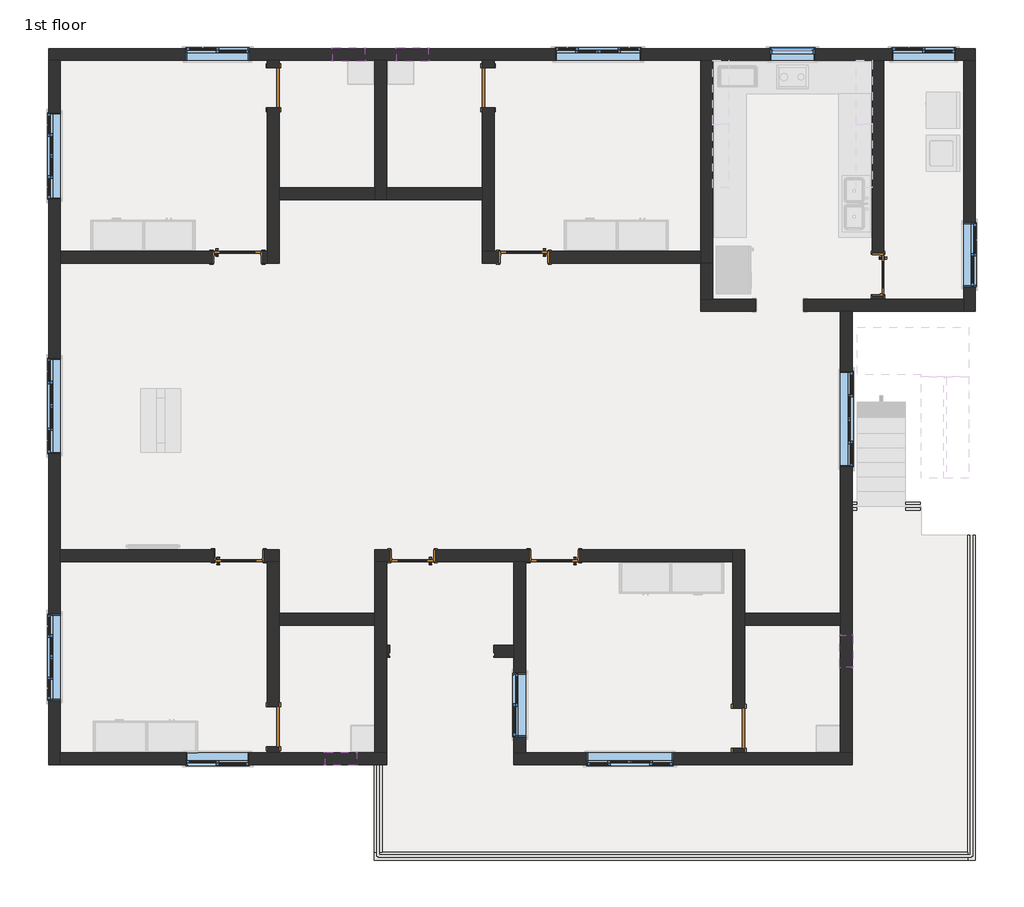
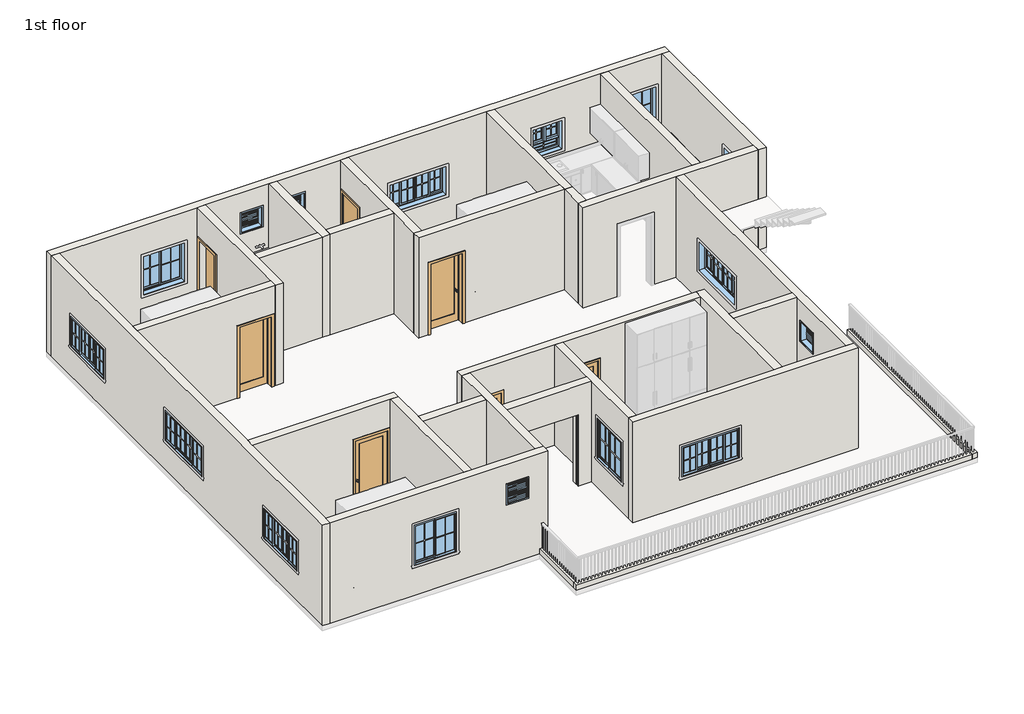
# One storey, part 1 of 4: 31 walls, 16 windows, 10 doors.
"""IFC4 building model written with IfcOpenShell, lengths in millimetres."""

from ifc_helpers import new_model, si_unit, frame, origin, place, context, project, spatial, polyline, outline, extrude, faceted_brep, transform, mapped, element, save
from components import door_ac3c0746, door_868ee8a9, door_3b97b8e7, door_c0815308, door_5e1232af, door_bb98abfd, window_ced37e8f, window_f2d8fef0, window_5af5dca6, window_95c4569f, window_58cce754

model = new_model("IFC4")

# Units and contexts
model_context = context("Model", 3, world=origin())
ifc_project = project(units=[si_unit("LENGTHUNIT", "METRE", prefix="MILLI")], contexts=[model_context])

# Site, building, storey
site = spatial("IfcSite", under=ifc_project)
building = spatial("IfcBuilding", under=site)
storey = spatial("IfcBuildingStorey", under=building, Name="1st floor", Elevation=3810.0)

# Doors
placement = place(None, origin())
door_shape = door_ac3c0746(model_context)
element("IfcDoor", 1, ObjectType="Door-Interior-Single-1_Panel-Wood : 30\" x 84\"", at=placement, inside=storey, context=model_context, shape_type="MappedRepresentation", body=[
    mapped(door_shape, transform((7861.3010838, 2743.2660813, 3810.0), x_axis=(0.0, -1.0, 0.0), y_axis=(1.0, 0.0, 0.0), z_axis=(0.0, 0.0, 1.0))),
])
door_2_shape = door_868ee8a9(model_context)
element("IfcDoor", 2, ObjectType="Door-Interior-Single-1_Panel-Wood : 36\" x 84\"", at=placement, inside=storey, context=model_context, shape_type="MappedRepresentation", body=[
    mapped(door_2_shape, transform((1076.3260838, 3076.6410813, 3810.0), x_axis=(-1.0, 0.0, 0.0), y_axis=(0.0, -1.0, 0.0), z_axis=(0.0, 0.0, 1.0))),
])
element("IfcDoor", 3, ObjectType="Door-Interior-Single-1_Panel-Wood : 36\" x 84\"", at=placement, inside=storey, context=model_context, shape_type="MappedRepresentation", body=[
    mapped(door_2_shape, transform((-4384.6739162, -2644.7089187, 3810.0), x_axis=(1.0, 0.0, 0.0), y_axis=(0.0, 1.0, 0.0), z_axis=(0.0, 0.0, 1.0))),
])
door_3_shape = door_3b97b8e7(model_context)
element("IfcDoor", 4, ObjectType="Door-Interior-Single-1_Panel-Wood : 36\" x 84\"", at=placement, inside=storey, context=model_context, shape_type="MappedRepresentation", body=[
    mapped(door_3_shape, transform((1660.5260838, -2644.7089187, 3810.0), x_axis=(-1.0, 0.0, 0.0), y_axis=(0.0, -1.0, 0.0), z_axis=(0.0, 0.0, 1.0))),
])
element("IfcDoor", 5, ObjectType="Door-Interior-Single-1_Panel-Wood : 36\" x 84\"", at=placement, inside=storey, context=model_context, shape_type="MappedRepresentation", body=[
    mapped(door_3_shape, transform((-4410.0739162, 3076.6410813, 3810.0), x_axis=(1.0, 0.0, 0.0), y_axis=(0.0, 1.0, 0.0), z_axis=(0.0, 0.0, 1.0))),
])
door_4_shape = door_c0815308(model_context)
element("IfcDoor", 6, ObjectType="Door-Interior-Single-Full Glass-Wood : 32\" x 84\"", at=placement, inside=storey, context=model_context, shape_type="MappedRepresentation", body=[
    mapped(door_4_shape, transform((-1057.2739162, -2644.7089187, 3810.0), x_axis=(-1.0, 0.0, 0.0), y_axis=(0.0, -1.0, 0.0), z_axis=(0.0, 0.0, 1.0))),
])
door_5_shape = door_5e1232af(model_context)
element("IfcDoor", 7, ObjectType="Single-Flush : 30\" x 84\"", at=placement, inside=storey, context=model_context, shape_type="MappedRepresentation", body=[
    mapped(door_5_shape, transform((-3724.2739162, 6324.6660813, 3810.0), x_axis=(0.0, 1.0, 0.0), y_axis=(-1.0, 0.0, 0.0), z_axis=(0.0, 0.0, 1.0))),
])
door_6_shape = door_bb98abfd(model_context)
element("IfcDoor", 8, ObjectType="Single-Flush : 30\" x 84\"", at=placement, inside=storey, context=model_context, shape_type="MappedRepresentation", body=[
    mapped(door_6_shape, transform((390.5260838, 6324.6660813, 3810.0), x_axis=(0.0, 1.0, 0.0), y_axis=(-1.0, 0.0, 0.0), z_axis=(0.0, 0.0, 1.0))),
])
element("IfcDoor", 9, ObjectType="Single-Flush : 30\" x 84\"", at=placement, inside=storey, context=model_context, shape_type="MappedRepresentation", body=[
    mapped(door_6_shape, transform((-3724.2739162, -5918.1339187, 3810.0), x_axis=(0.0, -1.0, 0.0), y_axis=(1.0, 0.0, 0.0), z_axis=(0.0, 0.0, 1.0))),
])
element("IfcDoor", 10, ObjectType="Single-Flush : 30\" x 84\"", at=placement, inside=storey, context=model_context, shape_type="MappedRepresentation", body=[
    mapped(door_6_shape, transform((5191.1260838, -5943.5339187, 3810.0), x_axis=(0.0, -1.0, 0.0), y_axis=(1.0, 0.0, 0.0), z_axis=(0.0, 0.0, 1.0))),
])

# Walls
element("IfcWall", 11, ObjectType="Generic - 6\"", at=placement, inside=storey, context=model_context, shape_type="Brep", body=[
    faceted_brep([(9572.6260838, -2247.8339187, 3810.0), (9572.6260838, -8318.4339187, 3810.0), (9572.6260838, -8470.8339187, 3810.0), (9572.6260838, -8470.8339187, 3962.4), (9572.6260838, -8318.4339187, 3962.4), (9572.6260838, -2247.8339187, 3962.4), (9725.0260838, -2247.8339187, 3810.0), (9725.0260838, -2247.8339187, 3962.4), (9725.0260838, -8470.8339187, 3962.4), (9725.0260838, -8470.8339187, 3810.0)], [[[0, 1, 2, 3, 4, 5]], [[6, 7, 8, 9]], [[2, 1, 0, 6, 9]], [[5, 4, 3, 8, 7]], [[0, 5, 7, 6]], [[3, 2, 9, 8]]]),
])
element("IfcWall", 12, ObjectType="Generic - 6\"", at=placement, inside=storey, context=model_context, shape_type="Brep", body=[
    faceted_brep([(9572.6260838, -8318.4339187, 3810.0), (-1641.4739162, -8318.4339187, 3810.0), (-1793.8739162, -8318.4339187, 3810.0), (-1793.8739162, -8318.4339187, 3962.4), (-1641.4739162, -8318.4339187, 3962.4), (9572.6260838, -8318.4339187, 3962.4), (9572.6260838, -8470.8339187, 3810.0), (9572.6260838, -8470.8339187, 3962.4), (-1793.8739162, -8470.8339187, 3962.4), (-1793.8739162, -8470.8339187, 3810.0)], [[[0, 1, 2, 3, 4, 5]], [[6, 7, 8, 9]], [[2, 1, 0, 6, 9]], [[5, 4, 3, 8, 7]], [[0, 5, 7, 6]], [[3, 2, 9, 8]]]),
])
element("IfcWall", 13, ObjectType="Generic - 6\"", at=placement, inside=storey, context=model_context, shape_type="SweptSolid", body=[
    extrude(outline(polyline([(-1641.4739162, -6642.0339187), (-1641.4739162, -8318.4339187), (-1793.8739162, -8318.4339187), (-1793.8739162, -6642.0339187), (-1641.4739162, -6642.0339187)])), frame((0.0, 0.0, 3810.0), z_axis=(0.0, 0.0, 1.0), x_axis=(1.0, 0.0, 0.0)), (0.0, 0.0, 1.0), 152.4),
])
element("IfcWall", 14, ObjectType="Generic - 6\"", at=placement, inside=storey, context=model_context, shape_type="SweptSolid", body=[
    extrude(outline(polyline([(7362.8260838, -1612.8339187), (7451.7260838, -1612.8339187), (7451.7260838, -1765.2339187), (7362.8260838, -1765.2339187), (7362.8260838, -1612.8339187)])), frame((0.0, 0.0, 3810.0), z_axis=(0.0, 0.0, 1.0), x_axis=(1.0, 0.0, 0.0)), (0.0, 0.0, 1.0), 152.4),
])
element("IfcWall", 15, ObjectType="Generic - 6\"", at=placement, inside=storey, context=model_context, shape_type="SweptSolid", body=[
    extrude(outline(polyline([(8391.5260838, -1612.8339187), (8670.9260838, -1612.8339187), (8670.9260838, -1765.2339187), (8391.5260838, -1765.2339187), (8391.5260838, -1612.8339187)])), frame((0.0, 0.0, 3810.0), z_axis=(0.0, 0.0, 1.0), x_axis=(1.0, 0.0, 0.0)), (0.0, 0.0, 1.0), 152.4),
])
element("IfcWall", 16, ObjectType="Generic - 9\"", at=placement, inside=storey, context=model_context, shape_type="Brep", body=[
    faceted_brep([(-8029.5739162, 6845.3660813, 3810.0), (-7800.9739162, 6845.3660813, 3810.0), (-3838.5739162, 6845.3660813, 3810.0), (-3609.9739162, 6845.3660813, 3810.0), (-1781.1739162, 6845.3660813, 3810.0), (-1552.5739162, 6845.3660813, 3810.0), (276.2260838, 6845.3660813, 3810.0), (504.8260838, 6845.3660813, 3810.0), (4467.2260838, 6845.3660813, 3810.0), (4695.8260838, 6845.3660813, 3810.0), (7743.8260838, 6845.3660813, 3810.0), (7972.4260838, 6845.3660813, 3810.0), (9496.4260838, 6845.3660813, 3810.0), (9725.0260838, 6845.3660813, 3810.0), (9725.0260838, 6845.3660813, 6858.0), (9496.4260838, 6845.3660813, 6858.0), (7972.4260838, 6845.3660813, 6858.0), (7743.8260838, 6845.3660813, 6858.0), (4695.8260838, 6845.3660813, 6858.0), (4467.2260838, 6845.3660813, 6858.0), (504.8260838, 6845.3660813, 6858.0), (276.2260838, 6845.3660813, 6858.0), (-1552.5739162, 6845.3660813, 6858.0), (-1781.1739162, 6845.3660813, 6858.0), (-3609.9739162, 6845.3660813, 6858.0), (-3838.5739162, 6845.3660813, 6858.0), (-7800.9739162, 6845.3660813, 6858.0), (-8029.5739162, 6845.3660813, 6858.0), (3324.2260838, 6845.3660813, 5638.8), (3324.2260838, 6845.3660813, 4724.4), (1673.2260838, 6845.3660813, 4724.4), (1673.2260838, 6845.3660813, 5638.8), (9344.0260838, 6845.3660813, 5943.6), (9344.0260838, 6845.3660813, 4724.4), (8124.8260838, 6845.3660813, 4724.4), (8124.8260838, 6845.3660813, 5943.6), (-2581.2739162, 6845.3660813, 6248.4), (-1971.6739162, 6845.3660813, 6248.4), (-1971.6739162, 6845.3660813, 5638.8), (-2581.2739162, 6845.3660813, 5638.8), (-1362.0739162, 6845.3660813, 6248.4), (-752.4739162, 6845.3660813, 6248.4), (-752.4739162, 6845.3660813, 5638.8), (-1362.0739162, 6845.3660813, 5638.8), (-4181.4739162, 6845.3660813, 5943.6), (-4181.4739162, 6845.3660813, 4724.4), (-5400.6739162, 6845.3660813, 4724.4), (-5400.6739162, 6845.3660813, 5943.6), (6651.6260838, 6845.3660813, 5867.4), (6651.6260838, 6845.3660813, 4953.0), (5788.0260838, 6845.3660813, 4953.0), (5788.0260838, 6845.3660813, 5867.4), (-8029.5739162, 7073.9660813, 3810.0), (-8029.5739162, 7073.9660813, 6858.0), (9725.0260838, 7073.9660813, 6858.0), (9725.0260838, 7073.9660813, 3810.0), (3324.2260838, 7073.9660813, 5638.8), (1673.2260838, 7073.9660813, 5638.8), (1673.2260838, 7073.9660813, 4724.4), (3324.2260838, 7073.9660813, 4724.4), (9344.0260838, 7073.9660813, 5943.6), (8124.8260838, 7073.9660813, 5943.6), (8124.8260838, 7073.9660813, 4724.4), (9344.0260838, 7073.9660813, 4724.4), (-2581.2739162, 7073.9660813, 6248.4), (-2581.2739162, 7073.9660813, 5638.8), (-1971.6739162, 7073.9660813, 5638.8), (-1971.6739162, 7073.9660813, 6248.4), (-1362.0739162, 7073.9660813, 6248.4), (-1362.0739162, 7073.9660813, 5638.8), (-752.4739162, 7073.9660813, 5638.8), (-752.4739162, 7073.9660813, 6248.4), (-4181.4739162, 7073.9660813, 5943.6), (-5400.6739162, 7073.9660813, 5943.6), (-5400.6739162, 7073.9660813, 4724.4), (-4181.4739162, 7073.9660813, 4724.4), (6651.6260838, 7073.9660813, 5867.4), (5788.0260838, 7073.9660813, 5867.4), (5788.0260838, 7073.9660813, 4953.0), (6651.6260838, 7073.9660813, 4953.0)], [[[0, 1, 2, 3, 4, 5, 6, 7, 8, 9, 10, 11, 12, 13, 14, 15, 16, 17, 18, 19, 20, 21, 22, 23, 24, 25, 26, 27], [28, 29, 30, 31], [32, 33, 34, 35], [36, 37, 38, 39], [40, 41, 42, 43], [44, 45, 46, 47], [48, 49, 50, 51]], [[52, 53, 54, 55], [56, 57, 58, 59], [60, 61, 62, 63], [64, 65, 66, 67], [68, 69, 70, 71], [72, 73, 74, 75], [76, 77, 78, 79]], [[13, 12, 11, 10, 9, 8, 7, 6, 5, 4, 3, 2, 1, 0, 52, 55]], [[0, 27, 53, 52]], [[14, 13, 55, 54]], [[29, 28, 56, 59]], [[30, 29, 59, 58]], [[31, 30, 58, 57]], [[28, 31, 57, 56]], [[33, 32, 60, 63]], [[34, 33, 63, 62]], [[35, 34, 62, 61]], [[32, 35, 61, 60]], [[65, 64, 36, 39]], [[66, 65, 39, 38]], [[67, 66, 38, 37]], [[64, 67, 37, 36]], [[69, 68, 40, 43]], [[70, 69, 43, 42]], [[71, 70, 42, 41]], [[68, 71, 41, 40]], [[45, 44, 72, 75]], [[46, 45, 75, 74]], [[47, 46, 74, 73]], [[44, 47, 73, 72]], [[49, 48, 76, 79]], [[50, 49, 79, 78]], [[51, 50, 78, 77]], [[48, 51, 77, 76]], [[27, 26, 25, 24, 23, 22, 21, 20, 19, 18, 17, 16, 15, 14, 54, 53]]]),
])
element("IfcWall", 17, ObjectType="Generic - 9\"", at=placement, inside=storey, context=model_context, shape_type="Brep", body=[
    faceted_brep([(-8029.5739162, 6845.3660813, 3810.0), (-8029.5739162, -6642.0339187, 3810.0), (-8029.5739162, -6642.0339187, 6858.0), (-8029.5739162, 6845.3660813, 6858.0), (-8029.5739162, 1143.0660813, 5638.8), (-8029.5739162, -685.7339187, 5638.8), (-8029.5739162, -685.7339187, 4724.4), (-8029.5739162, 1143.0660813, 4724.4), (-8029.5739162, 5842.0660813, 5638.8), (-8029.5739162, 4191.0660813, 5638.8), (-8029.5739162, 4191.0660813, 4724.4), (-8029.5739162, 5842.0660813, 4724.4), (-8029.5739162, -3759.1339187, 5638.8), (-8029.5739162, -5410.1339187, 5638.8), (-8029.5739162, -5410.1339187, 4724.4), (-8029.5739162, -3759.1339187, 4724.4), (-7800.9739162, 6845.3660813, 3810.0), (-7800.9739162, 6845.3660813, 6858.0), (-7800.9739162, 3187.7660813, 6858.0), (-7800.9739162, 2959.1660813, 6858.0), (-7800.9739162, -2527.2339187, 6858.0), (-7800.9739162, -2755.8339187, 6858.0), (-7800.9739162, -6413.4339187, 6858.0), (-7800.9739162, -6642.0339187, 6858.0), (-7800.9739162, -6642.0339187, 3810.0), (-7800.9739162, -6413.4339187, 3810.0), (-7800.9739162, -2755.8339187, 3810.0), (-7800.9739162, -2527.2339187, 3810.0), (-7800.9739162, 2959.1660813, 3810.0), (-7800.9739162, 3187.7660813, 3810.0), (-7800.9739162, 1143.0660813, 5638.8), (-7800.9739162, 1143.0660813, 4724.4), (-7800.9739162, -685.7339187, 4724.4), (-7800.9739162, -685.7339187, 5638.8), (-7800.9739162, 5842.0660813, 5638.8), (-7800.9739162, 5842.0660813, 4724.4), (-7800.9739162, 4191.0660813, 4724.4), (-7800.9739162, 4191.0660813, 5638.8), (-7800.9739162, -3759.1339187, 5638.8), (-7800.9739162, -3759.1339187, 4724.4), (-7800.9739162, -5410.1339187, 4724.4), (-7800.9739162, -5410.1339187, 5638.8)], [[[0, 1, 2, 3], [4, 5, 6, 7], [8, 9, 10, 11], [12, 13, 14, 15]], [[16, 17, 18, 19, 20, 21, 22, 23, 24, 25, 26, 27, 28, 29], [30, 31, 32, 33], [34, 35, 36, 37], [38, 39, 40, 41]], [[1, 0, 16, 29, 28, 27, 26, 25, 24]], [[0, 3, 17, 16]], [[2, 1, 24, 23]], [[31, 30, 4, 7]], [[32, 31, 7, 6]], [[33, 32, 6, 5]], [[30, 33, 5, 4]], [[35, 34, 8, 11]], [[36, 35, 11, 10]], [[37, 36, 10, 9]], [[34, 37, 9, 8]], [[39, 38, 12, 15]], [[40, 39, 15, 14]], [[41, 40, 14, 13]], [[38, 41, 13, 12]], [[3, 2, 23, 22, 21, 20, 19, 18, 17]]]),
])
element("IfcWall", 18, ObjectType="Generic - 9\"", at=placement, inside=storey, context=model_context, shape_type="Brep", body=[
    faceted_brep([(-3838.5739162, 6845.3660813, 6858.0), (-3838.5739162, 6845.3660813, 3810.0), (-3838.5739162, 6705.6660813, 3810.0), (-3838.5739162, 6705.6660813, 5943.6), (-3838.5739162, 5943.6660813, 5943.6), (-3838.5739162, 5943.6660813, 3810.0), (-3838.5739162, 3187.7660813, 3810.0), (-3838.5739162, 2959.1660813, 3810.0), (-3838.5739162, 2959.1660813, 6858.0), (-3838.5739162, 3187.7660813, 6858.0), (-3609.9739162, 6845.3660813, 3810.0), (-3609.9739162, 6845.3660813, 6858.0), (-3609.9739162, 4406.9660813, 6858.0), (-3609.9739162, 4178.3660813, 6858.0), (-3609.9739162, 2959.1660813, 6858.0), (-3609.9739162, 2959.1660813, 3810.0), (-3609.9739162, 4178.3660813, 3810.0), (-3609.9739162, 4406.9660813, 3810.0), (-3609.9739162, 5943.6660813, 3810.0), (-3609.9739162, 5943.6660813, 5943.6), (-3609.9739162, 6705.6660813, 5943.6), (-3609.9739162, 6705.6660813, 3810.0)], [[[0, 1, 2, 3, 4, 5, 6, 7, 8, 9]], [[10, 11, 12, 13, 14, 15, 16, 17, 18, 19, 20, 21]], [[1, 10, 21, 2]], [[15, 7, 6, 5, 18, 17, 16]], [[1, 0, 11, 10]], [[8, 7, 15, 14]], [[20, 3, 2, 21]], [[4, 19, 18, 5]], [[19, 4, 3, 20]], [[0, 9, 8, 14, 13, 12, 11]]]),
])
element("IfcWall", 19, ObjectType="Generic - 9\"", at=placement, inside=storey, context=model_context, shape_type="Brep", body=[
    faceted_brep([(-1781.1739162, 6845.3660813, 3810.0), (-1781.1739162, 4406.9660813, 3810.0), (-1781.1739162, 4178.3660813, 3810.0), (-1781.1739162, 4178.3660813, 6858.0), (-1781.1739162, 4406.9660813, 6858.0), (-1781.1739162, 6845.3660813, 6858.0), (-1552.5739162, 6845.3660813, 3810.0), (-1552.5739162, 6845.3660813, 6858.0), (-1552.5739162, 4406.9660813, 6858.0), (-1552.5739162, 4178.3660813, 6858.0), (-1552.5739162, 4178.3660813, 3810.0), (-1552.5739162, 4406.9660813, 3810.0)], [[[0, 1, 2, 3, 4, 5]], [[6, 7, 8, 9, 10, 11]], [[2, 1, 0, 6, 11, 10]], [[0, 5, 7, 6]], [[3, 2, 10, 9]], [[5, 4, 3, 9, 8, 7]]]),
])
element("IfcWall", 20, ObjectType="Generic - 9\"", at=placement, inside=storey, context=model_context, shape_type="Brep", body=[
    faceted_brep([(276.2260838, 6845.3660813, 6858.0), (276.2260838, 6845.3660813, 3810.0), (276.2260838, 6705.6660813, 3810.0), (276.2260838, 6705.6660813, 5943.6), (276.2260838, 5943.6660813, 5943.6), (276.2260838, 5943.6660813, 3810.0), (276.2260838, 4406.9660813, 3810.0), (276.2260838, 4178.3660813, 3810.0), (276.2260838, 3187.7660813, 3810.0), (276.2260838, 3187.7660813, 6858.0), (276.2260838, 4178.3660813, 6858.0), (276.2260838, 4406.9660813, 6858.0), (504.8260838, 6845.3660813, 3810.0), (504.8260838, 6845.3660813, 6858.0), (504.8260838, 3187.7660813, 6858.0), (504.8260838, 3187.7660813, 3810.0), (504.8260838, 5943.6660813, 3810.0), (504.8260838, 5943.6660813, 5943.6), (504.8260838, 6705.6660813, 5943.6), (504.8260838, 6705.6660813, 3810.0)], [[[0, 1, 2, 3, 4, 5, 6, 7, 8, 9, 10, 11]], [[12, 13, 14, 15, 16, 17, 18, 19]], [[1, 12, 19, 2]], [[15, 8, 7, 6, 5, 16]], [[1, 0, 13, 12]], [[9, 8, 15, 14]], [[18, 3, 2, 19]], [[4, 17, 16, 5]], [[17, 4, 3, 18]], [[0, 11, 10, 9, 14, 13]]]),
])
element("IfcWall", 21, ObjectType="Generic - 9\"", at=placement, inside=storey, context=model_context, shape_type="Brep", body=[
    faceted_brep([(4467.2260838, 6845.3660813, 3810.0), (4467.2260838, 3187.7660813, 3810.0), (4467.2260838, 2959.1660813, 3810.0), (4467.2260838, 2959.1660813, 6858.0), (4467.2260838, 3187.7660813, 6858.0), (4467.2260838, 6845.3660813, 6858.0), (4695.8260838, 6845.3660813, 3810.0), (4695.8260838, 6845.3660813, 6858.0), (4695.8260838, 2959.1660813, 6858.0), (4695.8260838, 2959.1660813, 3810.0)], [[[0, 1, 2, 3, 4, 5]], [[6, 7, 8, 9]], [[2, 1, 0, 6, 9]], [[3, 2, 9, 8]], [[0, 5, 7, 6]], [[5, 4, 3, 8, 7]]]),
])
element("IfcWall", 22, ObjectType="Generic - 9\"", at=placement, inside=storey, context=model_context, shape_type="SweptSolid", body=[
    extrude(outline(polyline([(3810.0, -3838.5739162), (6858.0, -3838.5739162), (6858.0, -7800.9739162), (3810.0, -7800.9739162), (3810.0, -4892.6739162), (5969.0, -4892.6739162), (5969.0, -3927.4739162), (3810.0, -3927.4739162), (3810.0, -3838.5739162)])), frame((0.0, 2959.1660813, 0.0), z_axis=(0.0, 1.0, 0.0), x_axis=(0.0, 0.0, 1.0)), (0.0, 0.0, 1.0), 228.6),
])
element("IfcWall", 23, ObjectType="Generic - 9\"", at=placement, inside=storey, context=model_context, shape_type="SweptSolid", body=[
    extrude(outline(polyline([(-3609.9739162, 4406.9660813), (-1781.1739162, 4406.9660813), (-1781.1739162, 4178.3660813), (-3609.9739162, 4178.3660813), (-3609.9739162, 4406.9660813)])), frame((0.0, 0.0, 3810.0), z_axis=(0.0, 0.0, 1.0), x_axis=(1.0, 0.0, 0.0)), (0.0, 0.0, 1.0), 3048.0),
])
element("IfcWall", 24, ObjectType="Generic - 9\"", at=placement, inside=storey, context=model_context, shape_type="SweptSolid", body=[
    extrude(outline(polyline([(276.2260838, 4178.3660813), (-1552.5739162, 4178.3660813), (-1552.5739162, 4406.9660813), (276.2260838, 4406.9660813), (276.2260838, 4178.3660813)])), frame((0.0, 0.0, 3810.0), z_axis=(0.0, 0.0, 1.0), x_axis=(1.0, 0.0, 0.0)), (0.0, 0.0, 1.0), 3048.0),
])
element("IfcWall", 25, ObjectType="Generic - 9\"", at=placement, inside=storey, context=model_context, shape_type="Brep", body=[
    faceted_brep([(4467.2260838, 2959.1660813, 3810.0), (4467.2260838, 2959.1660813, 6858.0), (276.2260838, 2959.1660813, 6858.0), (276.2260838, 2959.1660813, 3810.0), (593.7260838, 2959.1660813, 3810.0), (593.7260838, 2959.1660813, 5969.0), (1558.9260838, 2959.1660813, 5969.0), (1558.9260838, 2959.1660813, 3810.0), (4467.2260838, 3187.7660813, 6858.0), (4467.2260838, 3187.7660813, 3810.0), (1558.9260838, 3187.7660813, 3810.0), (1558.9260838, 3187.7660813, 5969.0), (593.7260838, 3187.7660813, 5969.0), (593.7260838, 3187.7660813, 3810.0), (504.8260838, 3187.7660813, 3810.0), (276.2260838, 3187.7660813, 3810.0), (276.2260838, 3187.7660813, 6858.0), (504.8260838, 3187.7660813, 6858.0)], [[[0, 1, 2, 3, 4, 5, 6, 7]], [[8, 9, 10, 11, 12, 13, 14, 15, 16, 17]], [[9, 0, 7, 10]], [[3, 15, 14, 13, 4]], [[1, 0, 9, 8]], [[3, 2, 16, 15]], [[12, 5, 4, 13]], [[5, 12, 11, 6]], [[6, 11, 10, 7]], [[2, 1, 8, 17, 16]]]),
])
element("IfcWall", 26, ObjectType="Generic - 9\"", at=placement, inside=storey, context=model_context, shape_type="Brep", body=[
    faceted_brep([(-7800.9739162, -2755.8339187, 6858.0), (-7800.9739162, -2755.8339187, 3810.0), (-4867.2739162, -2755.8339187, 3810.0), (-4867.2739162, -2755.8339187, 5969.0), (-3902.0739162, -2755.8339187, 5969.0), (-3902.0739162, -2755.8339187, 3810.0), (-3838.5739162, -2755.8339187, 3810.0), (-3609.9739162, -2755.8339187, 3810.0), (-3609.9739162, -2755.8339187, 6858.0), (-3838.5739162, -2755.8339187, 6858.0), (-7800.9739162, -2527.2339187, 3810.0), (-7800.9739162, -2527.2339187, 6858.0), (-3609.9739162, -2527.2339187, 6858.0), (-3609.9739162, -2527.2339187, 3810.0), (-3902.0739162, -2527.2339187, 3810.0), (-3902.0739162, -2527.2339187, 5969.0), (-4867.2739162, -2527.2339187, 5969.0), (-4867.2739162, -2527.2339187, 3810.0)], [[[0, 1, 2, 3, 4, 5, 6, 7, 8, 9]], [[10, 11, 12, 13, 14, 15, 16, 17]], [[1, 10, 17, 2]], [[13, 7, 6, 5, 14]], [[1, 0, 11, 10]], [[8, 7, 13, 12]], [[4, 15, 14, 5]], [[15, 4, 3, 16]], [[16, 3, 2, 17]], [[0, 9, 8, 12, 11]]]),
])
element("IfcWall", 27, ObjectType="Generic - 9\"", at=placement, inside=storey, context=model_context, shape_type="Brep", body=[
    faceted_brep([(-7800.9739162, -6642.0339187, 3810.0), (-1793.8739162, -6642.0339187, 3810.0), (-1641.4739162, -6642.0339187, 3810.0), (-1552.5739162, -6642.0339187, 3810.0), (-1552.5739162, -6642.0339187, 6858.0), (-1768.4739162, -6642.0339187, 6858.0), (-7800.9739162, -6642.0339187, 6858.0), (-5400.6739162, -6642.0339187, 4724.4), (-5400.6739162, -6642.0339187, 5943.6), (-4181.4739162, -6642.0339187, 5943.6), (-4181.4739162, -6642.0339187, 4724.4), (-2124.0739162, -6642.0339187, 6248.4), (-2124.0739162, -6642.0339187, 5638.8), (-2733.6739162, -6642.0339187, 5638.8), (-2733.6739162, -6642.0339187, 6248.4), (-1552.5739162, -6413.4339187, 3810.0), (-1781.1739162, -6413.4339187, 3810.0), (-3609.9739162, -6413.4339187, 3810.0), (-3838.5739162, -6413.4339187, 3810.0), (-7800.9739162, -6413.4339187, 3810.0), (-7800.9739162, -6413.4339187, 6858.0), (-3838.5739162, -6413.4339187, 6858.0), (-3609.9739162, -6413.4339187, 6858.0), (-1781.1739162, -6413.4339187, 6858.0), (-1552.5739162, -6413.4339187, 6858.0), (-5400.6739162, -6413.4339187, 5943.6), (-5400.6739162, -6413.4339187, 4724.4), (-4181.4739162, -6413.4339187, 4724.4), (-4181.4739162, -6413.4339187, 5943.6), (-2124.0739162, -6413.4339187, 5638.8), (-2124.0739162, -6413.4339187, 6248.4), (-2733.6739162, -6413.4339187, 6248.4), (-2733.6739162, -6413.4339187, 5638.8)], [[[0, 1, 2, 3, 4, 5, 6], [7, 8, 9, 10], [11, 12, 13, 14]], [[15, 16, 17, 18, 19, 20, 21, 22, 23, 24], [25, 26, 27, 28], [29, 30, 31, 32]], [[3, 2, 1, 0, 19, 18, 17, 16, 15]], [[0, 6, 20, 19]], [[25, 8, 7, 26]], [[26, 7, 10, 27]], [[27, 10, 9, 28]], [[8, 25, 28, 9]], [[12, 11, 30, 29]], [[13, 12, 29, 32]], [[14, 13, 32, 31]], [[11, 14, 31, 30]], [[3, 15, 24, 4]], [[24, 23, 22, 21, 20, 6, 5, 4]]]),
])
element("IfcWall", 28, ObjectType="Generic - 9\"", at=placement, inside=storey, context=model_context, shape_type="Brep", body=[
    faceted_brep([(-3609.9739162, -6413.4339187, 6858.0), (-3609.9739162, -6413.4339187, 3810.0), (-3609.9739162, -6299.1339187, 3810.0), (-3609.9739162, -6299.1339187, 5943.6), (-3609.9739162, -5537.1339187, 5943.6), (-3609.9739162, -5537.1339187, 3810.0), (-3609.9739162, -3975.0339187, 3810.0), (-3609.9739162, -3746.4339187, 3810.0), (-3609.9739162, -2755.8339187, 3810.0), (-3609.9739162, -2755.8339187, 6858.0), (-3609.9739162, -3746.4339187, 6858.0), (-3609.9739162, -3975.0339187, 6858.0), (-3838.5739162, -6413.4339187, 3810.0), (-3838.5739162, -6413.4339187, 6858.0), (-3838.5739162, -2755.8339187, 6858.0), (-3838.5739162, -2755.8339187, 3810.0), (-3838.5739162, -5537.1339187, 3810.0), (-3838.5739162, -5537.1339187, 5943.6), (-3838.5739162, -6299.1339187, 5943.6), (-3838.5739162, -6299.1339187, 3810.0)], [[[0, 1, 2, 3, 4, 5, 6, 7, 8, 9, 10, 11]], [[12, 13, 14, 15, 16, 17, 18, 19]], [[1, 12, 19, 2]], [[15, 8, 7, 6, 5, 16]], [[1, 0, 13, 12]], [[9, 8, 15, 14]], [[18, 3, 2, 19]], [[4, 17, 16, 5]], [[17, 4, 3, 18]], [[0, 11, 10, 9, 14, 13]]]),
])
element("IfcWall", 29, ObjectType="Generic - 9\"", at=placement, inside=storey, context=model_context, shape_type="Brep", body=[
    faceted_brep([(-1781.1739162, -2755.8339187, 3810.0), (-1781.1739162, -3746.4339187, 3810.0), (-1781.1739162, -3975.0339187, 3810.0), (-1781.1739162, -6413.4339187, 3810.0), (-1781.1739162, -6413.4339187, 6858.0), (-1781.1739162, -3975.0339187, 6858.0), (-1781.1739162, -3746.4339187, 6858.0), (-1781.1739162, -2755.8339187, 6858.0), (-1552.5739162, -2755.8339187, 3810.0), (-1552.5739162, -2755.8339187, 6858.0), (-1552.5739162, -4356.0339187, 6858.0), (-1552.5739162, -4584.6339187, 6858.0), (-1552.5739162, -6413.4339187, 6858.0), (-1552.5739162, -6413.4339187, 3810.0), (-1552.5739162, -4584.6339187, 3810.0), (-1552.5739162, -4356.0339187, 3810.0)], [[[0, 1, 2, 3, 4, 5, 6, 7]], [[8, 9, 10, 11, 12, 13, 14, 15]], [[3, 2, 1, 0, 8, 15, 14, 13]], [[0, 7, 9, 8]], [[7, 6, 5, 4, 12, 11, 10, 9]], [[3, 13, 12, 4]]]),
])
element("IfcWall", 30, ObjectType="Generic - 9\"", at=placement, inside=storey, context=model_context, shape_type="SweptSolid", body=[
    extrude(outline(polyline([(-3609.9739162, -3746.4339187), (-1781.1739162, -3746.4339187), (-1781.1739162, -3975.0339187), (-3609.9739162, -3975.0339187), (-3609.9739162, -3746.4339187)])), frame((0.0, 0.0, 3810.0), z_axis=(0.0, 0.0, 1.0), x_axis=(1.0, 0.0, 0.0)), (0.0, 0.0, 1.0), 3048.0),
])
element("IfcWall", 31, ObjectType="Generic - 9\"", at=placement, inside=storey, context=model_context, shape_type="Brep", body=[
    faceted_brep([(1114.4260838, -6413.4339187, 3810.0), (1114.4260838, -2755.8339187, 3810.0), (1114.4260838, -2755.8339187, 6858.0), (1114.4260838, -6413.4339187, 6858.0), (1114.4260838, -4889.4339187, 5943.6), (1114.4260838, -4889.4339187, 4724.4), (1114.4260838, -6108.6339187, 4724.4), (1114.4260838, -6108.6339187, 5943.6), (885.8260838, -2755.8339187, 3810.0), (885.8260838, -4356.0339187, 3810.0), (885.8260838, -4584.6339187, 3810.0), (885.8260838, -6413.4339187, 3810.0), (885.8260838, -6413.4339187, 6858.0), (885.8260838, -4584.6339187, 6858.0), (885.8260838, -4356.0339187, 6858.0), (885.8260838, -2755.8339187, 6858.0), (885.8260838, -4889.4339187, 4724.4), (885.8260838, -4889.4339187, 5943.6), (885.8260838, -6108.6339187, 5943.6), (885.8260838, -6108.6339187, 4724.4)], [[[0, 1, 2, 3], [4, 5, 6, 7]], [[8, 9, 10, 11, 12, 13, 14, 15], [16, 17, 18, 19]], [[1, 0, 11, 10, 9, 8]], [[2, 1, 8, 15]], [[0, 3, 12, 11]], [[4, 17, 16, 5]], [[5, 16, 19, 6]], [[6, 19, 18, 7]], [[17, 4, 7, 18]], [[3, 2, 15, 14, 13, 12]]]),
])
element("IfcWall", 32, ObjectType="Generic - 9\"", at=placement, inside=storey, context=model_context, shape_type="Brep", body=[
    faceted_brep([(-1781.1739162, -2527.2339187, 3810.0), (-1781.1739162, -2527.2339187, 6858.0), (5076.8260838, -2527.2339187, 6858.0), (5076.8260838, -2527.2339187, 3810.0), (2143.1260838, -2527.2339187, 3810.0), (2143.1260838, -2527.2339187, 5969.0), (1177.9260838, -2527.2339187, 5969.0), (1177.9260838, -2527.2339187, 3810.0), (-625.4739162, -2527.2339187, 3810.0), (-625.4739162, -2527.2339187, 5969.0), (-1489.0739162, -2527.2339187, 5969.0), (-1489.0739162, -2527.2339187, 3810.0), (-1781.1739162, -2755.8339187, 6858.0), (-1781.1739162, -2755.8339187, 3810.0), (-1552.5739162, -2755.8339187, 3810.0), (-1489.0739162, -2755.8339187, 3810.0), (-1489.0739162, -2755.8339187, 5969.0), (-625.4739162, -2755.8339187, 5969.0), (-625.4739162, -2755.8339187, 3810.0), (885.8260838, -2755.8339187, 3810.0), (1114.4260838, -2755.8339187, 3810.0), (1177.9260838, -2755.8339187, 3810.0), (1177.9260838, -2755.8339187, 5969.0), (2143.1260838, -2755.8339187, 5969.0), (2143.1260838, -2755.8339187, 3810.0), (5076.8260838, -2755.8339187, 3810.0), (5076.8260838, -2755.8339187, 6858.0), (1114.4260838, -2755.8339187, 6858.0), (885.8260838, -2755.8339187, 6858.0), (-1552.5739162, -2755.8339187, 6858.0)], [[[0, 1, 2, 3, 4, 5, 6, 7, 8, 9, 10, 11]], [[12, 13, 14, 15, 16, 17, 18, 19, 20, 21, 22, 23, 24, 25, 26, 27, 28, 29]], [[13, 0, 11, 15, 14]], [[3, 25, 24, 4]], [[7, 21, 20, 19, 18, 8]], [[1, 0, 13, 12]], [[3, 2, 26, 25]], [[6, 22, 21, 7]], [[22, 6, 5, 23]], [[23, 5, 4, 24]], [[10, 16, 15, 11]], [[16, 10, 9, 17]], [[17, 9, 8, 18]], [[2, 1, 12, 29, 28, 27, 26]]]),
])
element("IfcWall", 33, ObjectType="Generic - 9\"", at=placement, inside=storey, context=model_context, shape_type="Brep", body=[
    faceted_brep([(5305.4260838, -6413.4339187, 6858.0), (5305.4260838, -6413.4339187, 3810.0), (5305.4260838, -6324.5339187, 3810.0), (5305.4260838, -6324.5339187, 5943.6), (5305.4260838, -5562.5339187, 5943.6), (5305.4260838, -5562.5339187, 3810.0), (5305.4260838, -3975.0339187, 3810.0), (5305.4260838, -3746.4339187, 3810.0), (5305.4260838, -2527.2339187, 3810.0), (5305.4260838, -2527.2339187, 6858.0), (5305.4260838, -3746.4339187, 6858.0), (5305.4260838, -3975.0339187, 6858.0), (5076.8260838, -6413.4339187, 3810.0), (5076.8260838, -6413.4339187, 6858.0), (5076.8260838, -2755.8339187, 6858.0), (5076.8260838, -2527.2339187, 6858.0), (5076.8260838, -2527.2339187, 3810.0), (5076.8260838, -2755.8339187, 3810.0), (5076.8260838, -5562.5339187, 3810.0), (5076.8260838, -5562.5339187, 5943.6), (5076.8260838, -6324.5339187, 5943.6), (5076.8260838, -6324.5339187, 3810.0)], [[[0, 1, 2, 3, 4, 5, 6, 7, 8, 9, 10, 11]], [[12, 13, 14, 15, 16, 17, 18, 19, 20, 21]], [[1, 12, 21, 2]], [[16, 8, 7, 6, 5, 18, 17]], [[1, 0, 13, 12]], [[9, 8, 16, 15]], [[20, 3, 2, 21]], [[4, 19, 18, 5]], [[19, 4, 3, 20]], [[0, 11, 10, 9, 15, 14, 13]]]),
])
element("IfcWall", 34, ObjectType="Generic - 9\"", at=placement, inside=storey, context=model_context, shape_type="Brep", body=[
    faceted_brep([(7362.8260838, -6413.4339187, 3810.0), (7362.8260838, -1765.2339187, 3810.0), (7362.8260838, -1612.8339187, 3810.0), (7362.8260838, 2044.7660813, 3810.0), (7362.8260838, 2044.7660813, 6858.0), (7362.8260838, -1689.0339187, 6858.0), (7362.8260838, -6413.4339187, 6858.0), (7362.8260838, -939.7339187, 4724.4), (7362.8260838, -939.7339187, 5638.8), (7362.8260838, 889.0660813, 5638.8), (7362.8260838, 889.0660813, 4724.4), (7362.8260838, -4165.5339187, 6248.4), (7362.8260838, -4165.5339187, 5638.8), (7362.8260838, -4775.1339187, 5638.8), (7362.8260838, -4775.1339187, 6248.4), (7134.2260838, 2044.7660813, 3810.0), (7134.2260838, -3746.4339187, 3810.0), (7134.2260838, -3975.0339187, 3810.0), (7134.2260838, -6413.4339187, 3810.0), (7134.2260838, -6413.4339187, 6858.0), (7134.2260838, -3975.0339187, 6858.0), (7134.2260838, -3746.4339187, 6858.0), (7134.2260838, 2044.7660813, 6858.0), (7134.2260838, -939.7339187, 5638.8), (7134.2260838, -939.7339187, 4724.4), (7134.2260838, 889.0660813, 4724.4), (7134.2260838, 889.0660813, 5638.8), (7134.2260838, -4165.5339187, 5638.8), (7134.2260838, -4165.5339187, 6248.4), (7134.2260838, -4775.1339187, 6248.4), (7134.2260838, -4775.1339187, 5638.8)], [[[0, 1, 2, 3, 4, 5, 6], [7, 8, 9, 10], [11, 12, 13, 14]], [[15, 16, 17, 18, 19, 20, 21, 22], [23, 24, 25, 26], [27, 28, 29, 30]], [[3, 2, 1, 0, 18, 17, 16, 15]], [[4, 3, 15, 22]], [[0, 6, 19, 18]], [[23, 8, 7, 24]], [[24, 7, 10, 25]], [[25, 10, 9, 26]], [[8, 23, 26, 9]], [[12, 11, 28, 27]], [[13, 12, 27, 30]], [[14, 13, 30, 29]], [[11, 14, 29, 28]], [[22, 21, 20, 19, 6, 5, 4]]]),
])
element("IfcWall", 35, ObjectType="Generic - 9\"", at=placement, inside=storey, context=model_context, shape_type="SweptSolid", body=[
    extrude(outline(polyline([(5305.4260838, -3746.4339187), (7134.2260838, -3746.4339187), (7134.2260838, -3975.0339187), (5305.4260838, -3975.0339187), (5305.4260838, -3746.4339187)])), frame((0.0, 0.0, 3810.0), z_axis=(0.0, 0.0, 1.0), x_axis=(1.0, 0.0, 0.0)), (0.0, 0.0, 1.0), 3048.0),
])
element("IfcWall", 36, ObjectType="Generic - 9\"", at=placement, inside=storey, context=model_context, shape_type="SweptSolid", body=[
    extrude(outline(polyline([(6845.3660813, 6858.0), (6845.3660813, 3810.0), (3149.6660813, 3810.0), (3149.6660813, 5969.0), (2336.8660813, 5969.0), (2336.8660813, 3810.0), (2273.3660813, 3810.0), (2273.3660813, 6858.0), (6845.3660813, 6858.0)])), frame((7743.8260838, 0.0, 0.0), z_axis=(1.0, 0.0, 0.0), x_axis=(0.0, 1.0, 0.0)), (0.0, 0.0, 1.0), 228.6),
])
element("IfcWall", 37, ObjectType="Generic - 9\"", at=placement, inside=storey, context=model_context, shape_type="Brep", body=[
    faceted_brep([(4467.2260838, 2273.3660813, 3810.0), (4467.2260838, 2273.3660813, 6858.0), (4695.8260838, 2273.3660813, 6858.0), (7743.8260838, 2273.3660813, 6858.0), (7972.4260838, 2273.3660813, 6858.0), (9496.4260838, 2273.3660813, 6858.0), (9496.4260838, 2273.3660813, 3810.0), (7972.4260838, 2273.3660813, 3810.0), (7743.8260838, 2273.3660813, 3810.0), (6435.7260838, 2273.3660813, 3810.0), (6435.7260838, 2273.3660813, 5943.6), (5521.3260838, 2273.3660813, 5943.6), (5521.3260838, 2273.3660813, 3810.0), (4695.8260838, 2273.3660813, 3810.0), (4467.2260838, 2044.7660813, 6858.0), (4467.2260838, 2044.7660813, 3810.0), (5521.3260838, 2044.7660813, 3810.0), (5521.3260838, 2044.7660813, 5943.6), (6435.7260838, 2044.7660813, 5943.6), (6435.7260838, 2044.7660813, 3810.0), (7134.2260838, 2044.7660813, 3810.0), (7362.8260838, 2044.7660813, 3810.0), (9496.4260838, 2044.7660813, 3810.0), (9496.4260838, 2044.7660813, 6858.0), (7362.8260838, 2044.7660813, 6858.0), (7134.2260838, 2044.7660813, 6858.0)], [[[0, 1, 2, 3, 4, 5, 6, 7, 8, 9, 10, 11, 12, 13]], [[14, 15, 16, 17, 18, 19, 20, 21, 22, 23, 24, 25]], [[15, 0, 13, 12, 16]], [[6, 22, 21, 20, 19, 9, 8, 7]], [[1, 0, 15, 14]], [[18, 10, 9, 19]], [[11, 17, 16, 12]], [[10, 18, 17, 11]], [[5, 4, 3, 2, 1, 14, 25, 24, 23]], [[6, 5, 23, 22]]]),
])
element("IfcWall", 38, ObjectType="Generic - 9\"", at=placement, inside=storey, context=model_context, shape_type="SweptSolid", body=[
    extrude(outline(polyline([(4695.8260838, 2959.1660813), (4695.8260838, 2273.3660813), (4467.2260838, 2273.3660813), (4467.2260838, 2959.1660813), (4695.8260838, 2959.1660813)])), frame((0.0, 0.0, 3810.0), z_axis=(0.0, 0.0, 1.0), x_axis=(1.0, 0.0, 0.0)), (0.0, 0.0, 1.0), 3048.0),
])
element("IfcWall", 39, ObjectType="Generic - 9\"", at=placement, inside=storey, context=model_context, shape_type="Brep", body=[
    faceted_brep([(9496.4260838, 6845.3660813, 3810.0), (9496.4260838, 2273.3660813, 3810.0), (9496.4260838, 2044.7660813, 3810.0), (9496.4260838, 2044.7660813, 6858.0), (9496.4260838, 2273.3660813, 6858.0), (9496.4260838, 6845.3660813, 6858.0), (9496.4260838, 2514.6660813, 5943.6), (9496.4260838, 2514.6660813, 4724.4), (9496.4260838, 3733.8660813, 4724.4), (9496.4260838, 3733.8660813, 5943.6), (9725.0260838, 2044.7660813, 3810.0), (9725.0260838, 6845.3660813, 3810.0), (9725.0260838, 6845.3660813, 6858.0), (9725.0260838, 2044.7660813, 6858.0), (9725.0260838, 2514.6660813, 4724.4), (9725.0260838, 2514.6660813, 5943.6), (9725.0260838, 3733.8660813, 5943.6), (9725.0260838, 3733.8660813, 4724.4)], [[[0, 1, 2, 3, 4, 5], [6, 7, 8, 9]], [[10, 11, 12, 13], [14, 15, 16, 17]], [[2, 1, 0, 11, 10]], [[0, 5, 12, 11]], [[6, 15, 14, 7]], [[7, 14, 17, 8]], [[8, 17, 16, 9]], [[15, 6, 9, 16]], [[5, 4, 3, 13, 12]], [[3, 2, 10, 13]]]),
])
element("IfcWall", 40, ObjectType="Generic - 9\"", at=placement, inside=storey, context=model_context, shape_type="Brep", body=[
    faceted_brep([(885.8260838, -6642.0339187, 3810.0), (7362.8260838, -6642.0339187, 3810.0), (7362.8260838, -6642.0339187, 6858.0), (885.8260838, -6642.0339187, 6858.0), (2282.8260838, -6642.0339187, 4724.4), (2282.8260838, -6642.0339187, 5638.8), (3933.8260838, -6642.0339187, 5638.8), (3933.8260838, -6642.0339187, 4724.4), (7362.8260838, -6413.4339187, 3810.0), (7134.2260838, -6413.4339187, 3810.0), (5305.4260838, -6413.4339187, 3810.0), (5076.8260838, -6413.4339187, 3810.0), (1114.4260838, -6413.4339187, 3810.0), (885.8260838, -6413.4339187, 3810.0), (885.8260838, -6413.4339187, 6858.0), (1114.4260838, -6413.4339187, 6858.0), (5076.8260838, -6413.4339187, 6858.0), (5305.4260838, -6413.4339187, 6858.0), (7134.2260838, -6413.4339187, 6858.0), (7362.8260838, -6413.4339187, 6858.0), (2282.8260838, -6413.4339187, 5638.8), (2282.8260838, -6413.4339187, 4724.4), (3933.8260838, -6413.4339187, 4724.4), (3933.8260838, -6413.4339187, 5638.8)], [[[0, 1, 2, 3], [4, 5, 6, 7]], [[8, 9, 10, 11, 12, 13, 14, 15, 16, 17, 18, 19], [20, 21, 22, 23]], [[1, 0, 13, 12, 11, 10, 9, 8]], [[2, 1, 8, 19]], [[0, 3, 14, 13]], [[20, 5, 4, 21]], [[21, 4, 7, 22]], [[22, 7, 6, 23]], [[5, 20, 23, 6]], [[3, 2, 19, 18, 17, 16, 15, 14]]]),
])
element("IfcWall", 41, ObjectType="Generic - 9\"", at=placement, inside=storey, context=model_context, shape_type="Brep", body=[
    faceted_brep([(-1552.5739162, -4584.6339187, 6858.0), (-1552.5739162, -4584.6339187, 3810.0), (-1498.4739162, -4584.6339187, 3810.0), (-1498.4739162, -4584.6339187, 5979.5), (501.5260838, -4584.6339187, 5979.5), (501.5260838, -4584.6339187, 3810.0), (885.8260838, -4584.6339187, 3810.0), (885.8260838, -4584.6339187, 6858.0), (-1552.5739162, -4356.0339187, 3810.0), (-1552.5739162, -4356.0339187, 6858.0), (885.8260838, -4356.0339187, 6858.0), (885.8260838, -4356.0339187, 3810.0), (501.5260838, -4356.0339187, 3810.0), (501.5260838, -4356.0339187, 5979.5), (-1498.4739162, -4356.0339187, 5979.5), (-1498.4739162, -4356.0339187, 3810.0), (-1498.4739162, -4494.6339187, 3810.0), (-1513.4739162, -4494.6339187, 3810.0), (-1513.4739162, -4564.6339187, 3810.0), (-1498.4739162, -4564.6339187, 3810.0), (501.5260838, -4564.6339187, 3810.0), (516.5260838, -4564.6339187, 3810.0), (516.5260838, -4494.6339187, 3810.0), (501.5260838, -4494.6339187, 3810.0), (-1498.4739162, -4564.6339187, 5979.5), (501.5260838, -4564.6339187, 5979.5), (501.5260838, -4494.6339187, 5979.5), (-1498.4739162, -4494.6339187, 5979.5), (516.5260838, -4494.6339187, 5994.5), (-1513.4739162, -4494.6339187, 5994.5), (516.5260838, -4564.6339187, 5994.5), (-1513.4739162, -4564.6339187, 5994.5)], [[[0, 1, 2, 3, 4, 5, 6, 7]], [[8, 9, 10, 11, 12, 13, 14, 15]], [[1, 8, 15, 16, 17, 18, 19, 2]], [[11, 6, 5, 20, 21, 22, 23, 12]], [[1, 0, 9, 8]], [[7, 6, 11, 10]], [[24, 25, 4, 3]], [[26, 27, 14, 13]], [[27, 16, 15, 14]], [[23, 26, 13, 12]], [[27, 26, 23, 22, 28, 29, 17, 16]], [[28, 22, 21, 30]], [[25, 24, 19, 18, 31, 30, 21, 20]], [[25, 20, 5, 4]], [[19, 24, 3, 2]], [[17, 29, 31, 18]], [[29, 28, 30, 31]], [[0, 7, 10, 9]]]),
])

# Windows
window_shape = window_ced37e8f(model_context)
element("IfcWindow", 42, ObjectType="Window-Casement-Double-Awning : 34\" x 36\"", at=placement, inside=storey, context=model_context, shape_type="MappedRepresentation", body=[
    mapped(window_shape, transform((6219.8260838, 6959.6660813, 4038.6), x_axis=(1.0, 0.0, 0.0), y_axis=(0.0, 1.0, 0.0), z_axis=(0.0, 0.0, 1.0))),
])
window_2_shape = window_f2d8fef0(model_context)
element("IfcWindow", 43, ObjectType="Window-Louvers : 24\" x 24\"", at=placement, inside=storey, context=model_context, shape_type="MappedRepresentation", body=[
    mapped(window_2_shape, transform((-2276.4739162, 6966.0160813, 4724.4), x_axis=(1.0, 0.0, 0.0), y_axis=(0.0, 1.0, 0.0), z_axis=(0.0, 0.0, 1.0))),
])
element("IfcWindow", 44, ObjectType="Window-Louvers : 24\" x 24\"", at=placement, inside=storey, context=model_context, shape_type="MappedRepresentation", body=[
    mapped(window_2_shape, transform((-1057.2739162, 6966.0160813, 4724.4), x_axis=(1.0, 0.0, 0.0), y_axis=(0.0, 1.0, 0.0), z_axis=(0.0, 0.0, 1.0))),
])
element("IfcWindow", 45, ObjectType="Window-Louvers : 24\" x 24\"", at=placement, inside=storey, context=model_context, shape_type="MappedRepresentation", body=[
    mapped(window_2_shape, transform((-2428.8739162, -6534.0839187, 4724.4), x_axis=(-1.0, 0.0, 0.0), y_axis=(0.0, -1.0, 0.0), z_axis=(0.0, 0.0, 1.0))),
])
element("IfcWindow", 46, ObjectType="Window-Louvers : 24\" x 24\"", at=placement, inside=storey, context=model_context, shape_type="MappedRepresentation", body=[
    mapped(window_2_shape, transform((7254.8760838, -4470.3339187, 4724.4), x_axis=(0.0, -1.0, 0.0), y_axis=(1.0, 0.0, 0.0), z_axis=(0.0, 0.0, 1.0))),
])
window_3_shape = window_5af5dca6(model_context)
element("IfcWindow", 47, ObjectType="Window-Sliding-Double : 48\" x 48\"", at=placement, inside=storey, context=model_context, shape_type="MappedRepresentation", body=[
    mapped(window_3_shape, transform((996.3160838, -5499.0339187, 3810.0), x_axis=(0.0, 1.0, 0.0), y_axis=(-1.0, 0.0, 0.0), z_axis=(0.0, 0.0, 1.0))),
])
element("IfcWindow", 48, ObjectType="Window-Sliding-Double : 48\" x 48\"", at=placement, inside=storey, context=model_context, shape_type="MappedRepresentation", body=[
    mapped(window_3_shape, transform((8734.4260838, 6963.4760813, 3810.0), x_axis=(1.0, 0.0, 0.0), y_axis=(0.0, 1.0, 0.0), z_axis=(0.0, 0.0, 1.0))),
])
element("IfcWindow", 49, ObjectType="Window-Sliding-Double : 48\" x 48\"", at=placement, inside=storey, context=model_context, shape_type="MappedRepresentation", body=[
    mapped(window_3_shape, transform((9614.5360838, 3124.2660813, 3810.0), x_axis=(0.0, -1.0, 0.0), y_axis=(1.0, 0.0, 0.0), z_axis=(0.0, 0.0, 1.0))),
])
element("IfcWindow", 50, ObjectType="Window-Sliding-Double : 48\" x 48\"", at=placement, inside=storey, context=model_context, shape_type="MappedRepresentation", body=[
    mapped(window_3_shape, transform((-4791.0739162, -6531.5439187, 3810.0), x_axis=(-1.0, 0.0, 0.0), y_axis=(0.0, -1.0, 0.0), z_axis=(0.0, 0.0, 1.0))),
])
element("IfcWindow", 51, ObjectType="Window-Sliding-Double : 48\" x 48\"", at=placement, inside=storey, context=model_context, shape_type="MappedRepresentation", body=[
    mapped(window_3_shape, transform((-4791.0739162, 6963.4760813, 3810.0), x_axis=(1.0, 0.0, 0.0), y_axis=(0.0, 1.0, 0.0), z_axis=(0.0, 0.0, 1.0))),
])
window_4_shape = window_95c4569f(model_context)
element("IfcWindow", 52, ObjectType="Window-Sliding-Four : 65\" x 36\"", at=placement, inside=storey, context=model_context, shape_type="MappedRepresentation", body=[
    mapped(window_4_shape, transform((2498.7260838, 6963.4760813, 3810.0), x_axis=(1.0, 0.0, 0.0), y_axis=(0.0, 1.0, 0.0), z_axis=(0.0, 0.0, 1.0))),
])
element("IfcWindow", 53, ObjectType="Window-Sliding-Four : 65\" x 36\"", at=placement, inside=storey, context=model_context, shape_type="MappedRepresentation", body=[
    mapped(window_4_shape, transform((3108.3260838, -6531.5439187, 3810.0), x_axis=(-1.0, 0.0, 0.0), y_axis=(0.0, -1.0, 0.0), z_axis=(0.0, 0.0, 1.0))),
])
element("IfcWindow", 54, ObjectType="Window-Sliding-Four : 65\" x 36\"", at=placement, inside=storey, context=model_context, shape_type="MappedRepresentation", body=[
    mapped(window_4_shape, transform((-7919.0839162, 5016.5660813, 3810.0), x_axis=(0.0, 1.0, 0.0), y_axis=(-1.0, 0.0, 0.0), z_axis=(0.0, 0.0, 1.0))),
])
element("IfcWindow", 55, ObjectType="Window-Sliding-Four : 65\" x 36\"", at=placement, inside=storey, context=model_context, shape_type="MappedRepresentation", body=[
    mapped(window_4_shape, transform((-7919.0839162, -4584.6339187, 3810.0), x_axis=(0.0, 1.0, 0.0), y_axis=(-1.0, 0.0, 0.0), z_axis=(0.0, 0.0, 1.0))),
])
window_5_shape = window_58cce754(model_context)
element("IfcWindow", 56, ObjectType="Window-Sliding-Four : 72\" x 36\"", at=placement, inside=storey, context=model_context, shape_type="MappedRepresentation", body=[
    mapped(window_5_shape, transform((-7919.0839162, 228.6660813, 3810.0), x_axis=(0.0, 1.0, 0.0), y_axis=(-1.0, 0.0, 0.0), z_axis=(0.0, 0.0, 1.0))),
])
element("IfcWindow", 57, ObjectType="Window-Sliding-Four : 72\" x 36\"", at=placement, inside=storey, context=model_context, shape_type="MappedRepresentation", body=[
    mapped(window_5_shape, transform((7252.3360838, -25.3339187, 3810.0), x_axis=(0.0, -1.0, 0.0), y_axis=(1.0, 0.0, 0.0), z_axis=(0.0, 0.0, 1.0))),
])

save(model, "model.ifc")

# Revit data of these elements
# Type "Door-Interior-Single-1_Panel-Wood : 30\" x 84\""
#   Type Mark = "11"
#   Assembly Code = "C1020300"
#   Analytic Construction = "Wooden"
#   Top Rail = 0' - 4 11/16"
#   Thickness = 0' - 1 3/8"
#   Thermal Resistance (R) = 2.5876 (h·ft²·°F)/BTU
#   Swing Angle [instance default] = 90.00°
#   Stiles = 0' - 4 3/4"
#   Rough Width = 2' - 8"
#   Rough Height = 7' - 1"
#   Height = 7' - 0"
#   Width = 2' - 6"
#   Heat Transfer Coefficient (U) = 0.3865 BTU/(h·ft²·°F)
#   Bottom Rail = 0' - 9 1/8"
#   Trim Material = Cherry
#   Panel Material = Cherry
#   Frame Material = Cherry
#   Door Handle Material = Aluminum
#   Visual Light Transmittance = 0
#   Solar Heat Gain Coefficient = 0
#   Wall Closure = (empty or 0)
#   Function = (empty or 0)
# Type "Door-Interior-Single-1_Panel-Wood : 36\" x 84\""
#   Type Mark = "8"
#   Assembly Code = "C1020300"
#   Analytic Construction = "Wooden"
#   Top Rail = 0' - 4 11/16"
#   Thickness = 0' - 1 3/8"
#   Thermal Resistance (R) = 2.5876 (h·ft²·°F)/BTU
#   Swing Angle [instance default] = 90.00°
#   Stiles = 0' - 4 3/4"
#   Rough Width = 3' - 2"
#   Rough Height = 7' - 1"
#   Height = 7' - 0"
#   Width = 3' - 0"
#   Heat Transfer Coefficient (U) = 0.3865 BTU/(h·ft²·°F)
#   Bottom Rail = 0' - 9 1/8"
#   Trim Material = Cherry
#   Panel Material = Cherry
#   Frame Material = Cherry
#   Door Handle Material = Aluminum
#   Visual Light Transmittance = 0
#   Solar Heat Gain Coefficient = 0
#   Wall Closure = (empty or 0)
#   Function = (empty or 0)
# Type "Door-Interior-Single-Full Glass-Wood : 32\" x 84\""
#   Type Mark = "9"
#   Assembly Code = "C1020300"
#   Analytic Construction = "Wood frame with single clear glass"
#   Top Rail = 0' - 4 11/16"
#   Thickness = 0' - 1 3/8"
#   Thermal Resistance (R) = 1.0102 (h·ft²·°F)/BTU
#   Swing Angle [instance default] = 90.00°
#   Stiles = 0' - 4 3/4"
#   Rough Width = 2' - 10"
#   Rough Height = 7' - 1"
#   Height = 7' - 0"
#   Width = 2' - 8"
#   Heat Transfer Coefficient (U) = 0.9900 BTU/(h·ft²·°F)
#   Bottom Rail = 0' - 9 1/8"
#   Show Grill [instance default] = yes
#   Trim Material = Cherry
#   Panel Material = Cherry
#   Frame Material = Cherry
#   Door Handle Material = Aluminum
#   Visual Light Transmittance = 0
#   Solar Heat Gain Coefficient = 0
#   Wall Closure = (empty or 0)
#   Function = (empty or 0)
# Type "Single-Flush : 30\" x 84\""
#   Type Mark = "4"
#   Construction Type Id = "MDOOR"
#   Assembly Code = "C1020"
#   Analytic Construction = "Metal"
#   Thickness = 0' - 2"
#   Heat Transfer Coefficient (U) = 0.651978 BTU/(h·ft²·°F)
#   Height = 7' - 0"
#   Trim Projection Ext = 0' - 1"
#   Trim Projection Int = 0' - 1"
#   Trim Width = 0' - 3"
#   Width = 2' - 6"
#   Define Thermal Properties by = 1
#   Define Thermal Properties by = 1
#   Door Material = Door - Panel
#   Frame Material = Door - Frame
#   Visual Light Transmittance = 0
#   Solar Heat Gain Coefficient = 0
#   Function = (empty or 0)
#   Wall Closure = (empty or 0)
# Type "Generic - 6\""
#   Assembly Code = "B2010"
#   Layers, outside or top first: 0' - 6" no material (function 1)
# Type "Generic - 9\""
#   Assembly Code = "B2010"
#   Layers, outside or top first: 0' - 9" no material (function 1)
# Type "Window-Casement-Double-Awning : 34\" x 36\""
#   Type Mark = "26"
#   Fire Rating = "0.5h"
#   Assembly Code = "B2020100"
#   Analytic Construction = "Double glazing - domestic"
#   Window Inset [instance default] = 0' - 0"
#   Wall Thickness [instance default] = 0' - 6"
#   Interior Wall Closure [instance default] = 0' - 2 1/4"
#   Half Width = 1' - 5"
#   Visual Light Transmittance = 0.81
#   Thermal Resistance (R) = 1.8146 (h·ft²·°F)/BTU
#   Solar Heat Gain Coefficient = 0.76
#   Rough Width = 2' - 10 1/2"
#   Rough Height = 3' - 0 1/2"
#   Open Window Height = 2' - 0"
#   Height = 3' - 0"
#   Heat Transfer Coefficient (U) = 0.5511 BTU/(h·ft²·°F)
#   Frame Extension [instance default] = 0' - 0 1/4"
#   Exterior Wall Closure [instance default] = 0' - 1 1/4"
#   Awning Height = 1' - 0"
#   Extension Jamb [instance default] = 0' - 2 1/4"
#   Default Sill Height = 3' - 0"
#   Width = 2' - 10"
#   Top Muntin Visibility = yes
#   Interior Trim Visibility [instance default] = yes
#   Bottom Muntin Visibility = yes
#   Exterior Trim Visibility [instance default] = yes
#   Extension Jamb Visibility [instance default] = yes
#   Interior Trim Material = Wood - Stained
#   Muntin Pattern = Muntin Pattern_2x2 : Muntin Pattern_2x2
#   Interior Trim = Trim-Window-Interior-Flat : Picture Frame
#   Interior Frame Material = Wood - Stained
#   Exterior Trim Material = Clad - White
#   Glass Panel Material = Glass
#   Exterior Trim = Trim-Window-Exterior-Flat : with Sill
#   Exterior Frame Material = Clad - White
#   Wall Closure = (empty or 0)
# Type "Window-Louvers : 24\" x 24\""
#   Type Mark = "24"
#   Construction Type Id = "GSP4R"
#   Assembly Code = "B20"
#   Analytic Construction = "1/8 in Pilkington single glazing"
#   Visual Light Transmittance = 0.9
#   Thermal Resistance (R) = 1.53941 (h·ft²·°F)/BTU
#   Solar Heat Gain Coefficient = 0.78
#   Max Height = 1' - 11.74264"
#   Height = 2' - 0"
#   Heat Transfer Coefficient (U) = 0.6496 BTU/(h·ft²·°F)
#   Blade Width [instance default] = 1' - 10 1/2"
#   Blade Vertical Thickness = 0' - 0.35355"
#   Blade Thickness = 0' - 0 1/4"
#   Blade Spacing = 0' - 1 1/2"
#   Blade Height = 0' - 1.85355"
#   Blade Depth = 0' - 3"
#   Blade Angle = 45.00°
#   Default Sill Height = 3' - 0"
#   Trim Projection_Exterior = 0' - 0 1/2"
#   Trim Projection_Interior = 0' - 0 1/2"
#   Trim Width_Exterior = 0' - 1 1/2"
#   Trim Width_Interior = 0' - 1 1/2"
#   Width = 2' - 0"
#   Max Blade Count = 12
#   Define Thermal Properties by = 1
#   Blade Count = 12
#   Frame Material = Birch
#   Louver Material = Birch
#   Trim Exterior Material = Birch
#   Trim Interior Material = Birch
#   Wall Closure = (empty or 0)
# Type "Window-Sliding-Double : 48\" x 48\""
#   Type Mark = "23"
#   Fire Rating = "0.5h"
#   Assembly Code = "B2020100"
#   Analytic Construction = "Double glazing - domestic"
#   Window Inset [instance default] = 0' - 0"
#   Wall Thickness [instance default] = 0' - 6"
#   Visual Light Transmittance = 0.81
#   Thermal Resistance (R) = 1.8146 (h·ft²·°F)/BTU
#   Solar Heat Gain Coefficient = 0.76
#   Muntin Width = 1' - 8 5/8"
#   Muntin Height = 3' - 6 1/4"
#   Interior Wall Closure [instance default] = 0' - 2 3/4"
#   Heat Transfer Coefficient (U) = 0.5511 BTU/(h·ft²·°F)
#   Frame Extension [instance default] = 0' - 0 1/4"
#   Exterior Wall Closure [instance default] = 0' - 1 1/4"
#   Rough Width = 4' - 0 1/2"
#   Rough Height = 4' - 0 1/2"
#   Height = 4' - 0"
#   Extension Jamb [instance default] = 0' - 2 3/4"
#   Default Sill Height = 3' - 0"
#   Width = 4' - 0"
#   Interior Trim Visibility [instance default] = yes
#   Indicator Visibility [instance default] = yes
#   Exterior Trim Visibility [instance default] = yes
#   Muntin Visibility = yes
#   Extension Jamb Visibility [instance default] = yes
#   Muntin Pattern = Muntin Pattern_2x2 : Muntin Pattern_2x2
#   Interior Trim Material = Wood - Stained
#   Interior Trim = Trim-Window-Interior-Flat : Picture Frame
#   Interior Frame Material = Wood - Stained
#   Glass Panel Material = Glass
#   Exterior Trim Material = Clad - White
#   Exterior Trim = Trim-Window-Exterior-Flat : with Sill
#   Exterior Frame Material = Clad - White
#   Wall Closure = (empty or 0)
# Type "Window-Sliding-Four : 65\" x 36\""
#   Type Mark = "19"
#   Fire Rating = "0.5h"
#   Assembly Code = "B2020100"
#   Analytic Construction = "Double glazing - domestic"
#   Window Inset [instance default] = 0' - 0"
#   Wall Thickness [instance default] = 0' - 6"
#   Visual Light Transmittance = 0.81
#   Thermal Resistance (R) = 1.8146 (h·ft²·°F)/BTU
#   Solar Heat Gain Coefficient = 0.76
